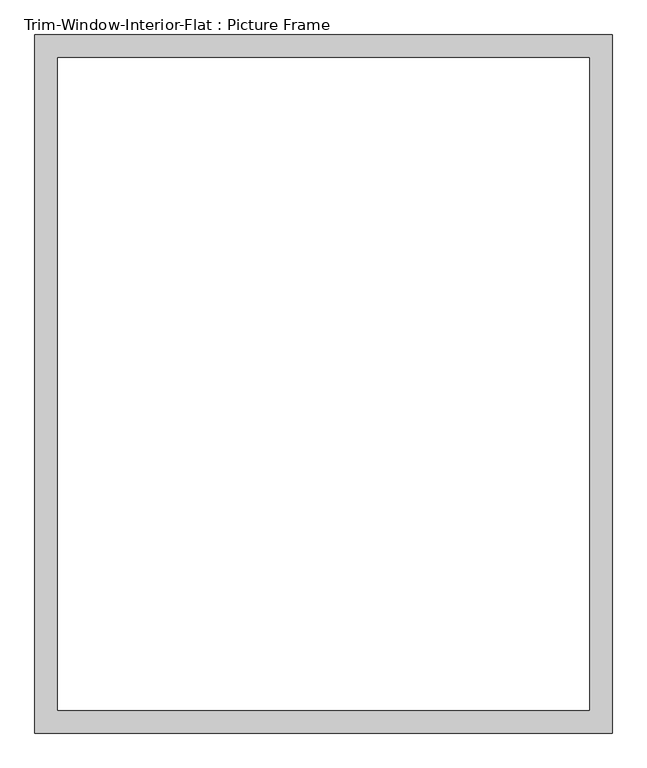
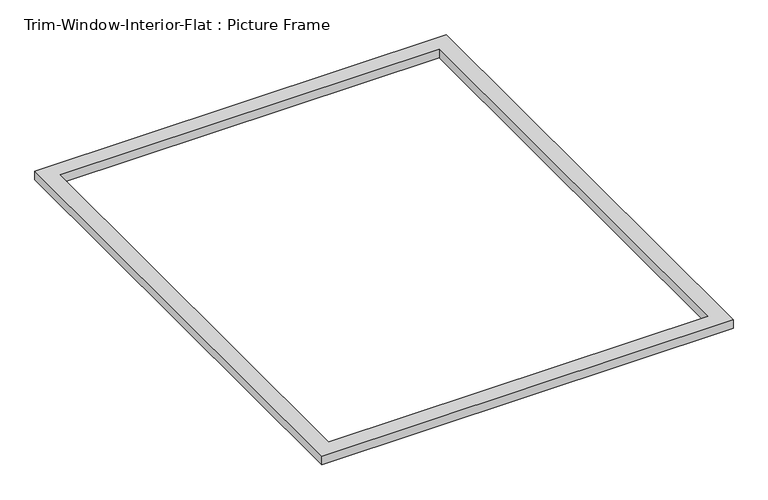
"""IFC4 building model written with IfcOpenShell, lengths in millimetres: proxy geometry, Trim-Window-Interior-Flat : Picture Frame."""

from ifc_helpers import new_model, si_unit, origin, origin_with_axes, place, context, project, spatial, polyline, outline, extrude, source, transform, mapped, element, save


def trim_window_interior_flat_picture_frame_717249e1(model_context):
    return source(origin(), model_context, "Body", "SweptSolid", [
        extrude(outline(polyline([(730.25, 44.45), (730.25, -1720.85), (-730.25, -1720.85), (-730.25, 44.45), (730.25, 44.45)]), holes=[polyline([(673.1, -12.7), (-673.1, -12.7), (-673.1, -1663.7), (673.1, -1663.7), (673.1, -12.7)])]), origin_with_axes(), (0.0, 0.0, 1.0), 31.75),
    ])


if __name__ == "__main__":
    model = new_model("IFC4")
    model_context = context("Model", 3, world=origin())
    ifc_project = project(units=[si_unit("LENGTHUNIT", "METRE", prefix="MILLI")], contexts=[model_context])
    site = spatial("IfcSite", under=ifc_project)
    building = spatial("IfcBuilding", under=site)
    placement = place(None, origin())
    trim_window_interior_flat_picture_frame_shape = trim_window_interior_flat_picture_frame_717249e1(model_context)
    element("IfcBuildingElementProxy", 1, Name="Trim-Window-Interior-Flat : Picture Frame", ObjectType="Trim-Window-Interior-Flat : Picture Frame", at=placement, inside=building, context=model_context, shape_type="MappedRepresentation", body=[
        mapped(trim_window_interior_flat_picture_frame_shape, transform((0.0, 0.0, 0.0), x_axis=(1.0, 0.0, 0.0), y_axis=(0.0, 1.0, 0.0), z_axis=(0.0, 0.0, 1.0))),
    ])
    save(model, "model.ifc")

# Revit data of these elements
# Type "Trim-Window-Interior-Flat : Picture Frame"
#   Trim Thickness_Picture Frame = 0' - 1 1/4"
#   Trim Width = 0' - 2 1/4"
#   Trim Thickness_with Sill = 0' - 0 3/4"
#   Sill Thickness = 0' - 1 1/4"
#   Opening Width [instance default] = 2' - 0"
#   Opening Height [instance default] = 3' - 0"
#   Default Elevation = 4' - 0"
#   Sill = no
#   Picture Frame = yes
#   Trim Material [instance default] = none
# Element 1 (IfcBuildingElementProxy, "Trim-Window-Interior-Flat : Picture Frame")
#   Opening Width = 4' - 6"
#   Opening Height = 5' - 6"
#   Trim Material = Wood - Stained
#   Materials on its faces: "Wood - Stained"
# Materials
#   "Wood - Stained": class "Wood", colour RGB 224 178 126, transparency 0, Cost = 0
